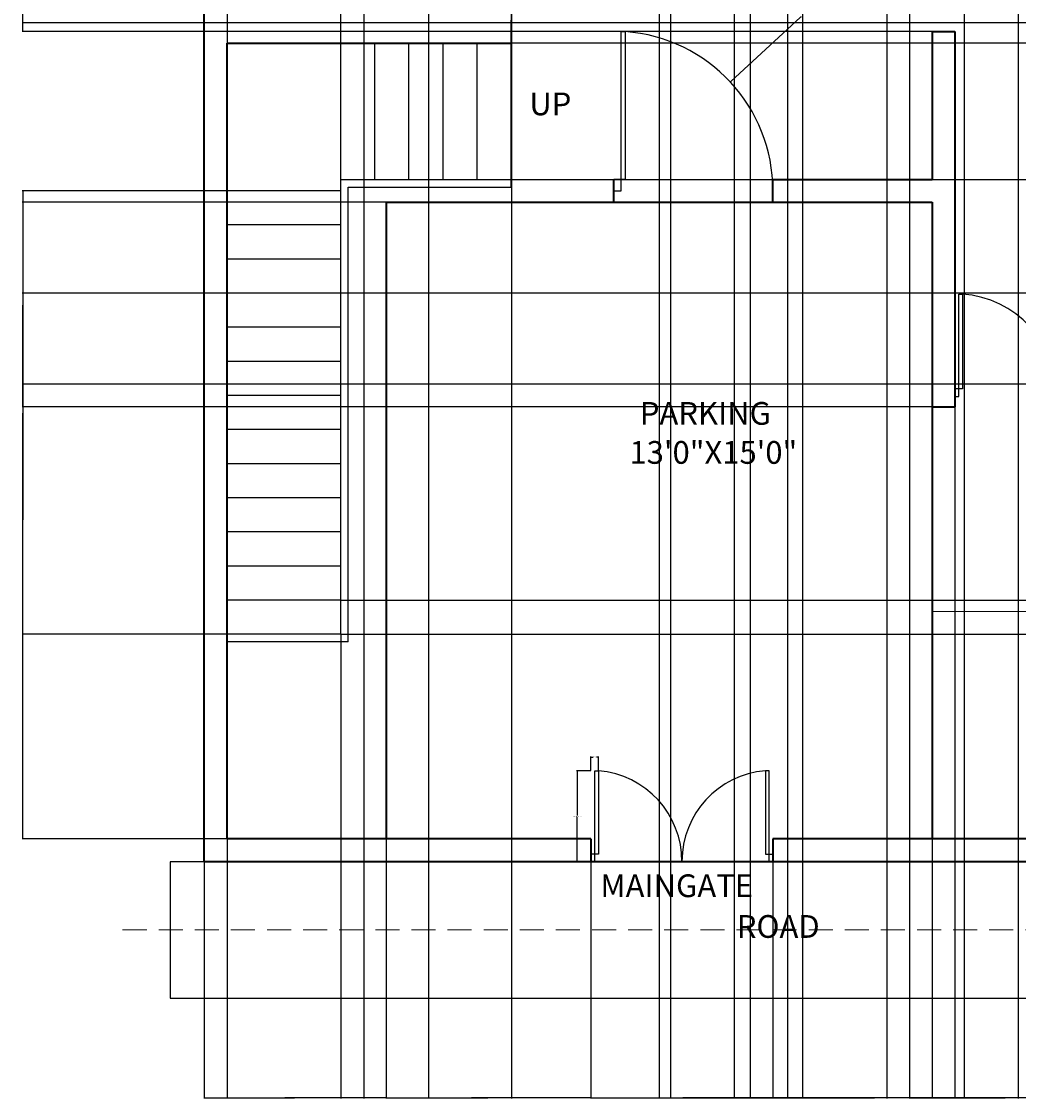
# Model space of a CAD drawing. Units: inches. Extents: x 2608 to 3003, y 1827 to 2396.
# Tile 1 of 5: x 2608 to 2871, y 1827 to 2111. Entities that reach past the tile are written whole.
import ezdxf

# ---------------------------------------------------------------- set-up
doc = ezdxf.new("R2010")
doc.units = ezdxf.units.IN
doc.linetypes.add('DASHED2', pattern=[9.525, 6.35, -3.175])
for name, color, linetype, lineweight in [('A-ANNO-DIMS', 2, 'Continuous', 18), ('A-ANNO-TEXT', 7, 'Continuous', 25), ('A-AREA-IDEN', 7, 'Continuous', 25), ('A-DOOR', 50, 'Continuous', 25), ('A-DOOR-GATE', 50, 'Continuous', 25), ('A-FLOR', 111, 'Continuous', 18), ('A-FLOR-STRS', 111, 'Continuous', 25), ('A-WALL', 111, 'Continuous', 35), ('C-ROAD', 111, 'Continuous', 25), ('C-ROAD-CNTR', 255, 'DASHED2', 18)]:
    doc.layers.add(name, color=color, linetype=linetype, lineweight=lineweight)
doc.styles.get("Standard").update_dxf_attribs({"font": 'arial.ttf'})
doc.dimstyles.get("Standard").update_dxf_attribs({"dimtxt": 0.18, "dimasz": 0.18, "dimexe": 0.18, "dimexo": 0.0625, "dimgap": 0.09, "dimtad": 0, "dimtih": 1, "dimtoh": 1, "dimdec": 4, "dimzin": 0, "dimdsep": 46, "dimtxsty": 'Standard', "dimcen": 0.09, "dimadec": 0, "dimazin": 0, "dimtfac": 1, "dimtdec": 4, "dimtofl": 0, "dimtmove": 0, "dimatfit": 3, "dimfxl": 1, "dimtolj": 1, "dimtzin": 0, "dimarcsym": 0})

# ---------------------------------------------------------------- blocks, each defined once
blk = doc.blocks.new('GATE-LEAF-24')
for p, q in [((1, 0), (1, 24)), ((1, 24), (2, 24)), ((2, 24), (2, 2)), ((2, 2), (0, 2)), ((0, 0), (1, 0))]:
    blk.add_line(p, q)
blk = doc.blocks.new('*D26')
at = {"layer": 'A-ANNO-DIMS', "color": 0, "lineweight": -2, "transparency": 16777216}
for p, q in [((2757.85, 1913.49), (2754.14, 1913.49)), ((2754.32, 1913.31), (2754.32, 1901.67)), ((2754.32, 1889.67), (2754.32, 1901.31)), ((2757.85, 1889.49), (2754.14, 1889.49))]:
    blk.add_line(p, q, dxfattribs=at)
at = {"layer": 'A-ANNO-DIMS', "color": 0, "transparency": 16777216}
for points in [[(2754.29, 1913.31), (2754.35, 1913.31), (2754.32, 1913.49)], [(2754.29, 1889.67), (2754.35, 1889.67), (2754.32, 1889.49)]]:
    blk.add_solid(points, dxfattribs=at)
at = {"layer": 'Defpoints', "color": 0, "transparency": 16777216}
for p in [(2754.32, 1913.49), (2757.92, 1913.49), (2757.92, 1889.49)]:
    blk.add_point(p, dxfattribs=at)
at = {"layer": 'A-ANNO-DIMS', "color": 0, "transparency": 16777216, "insert": (2754.32, 1901.49), "char_height": 0.18, "attachment_point": 5}
blk.add_mtext('\\A1;GATE LEAF 24 TYP.', dxfattribs=at)
blk = doc.blocks.new('*D27')
at = {"layer": 'A-ANNO-DIMS', "color": 0, "lineweight": -2, "transparency": 16777216}
for p, q in [((2757.92, 1913.55), (2757.92, 1917.27)), ((2758.1, 1917.09), (2758.46, 1917.09)), ((2759.74, 1917.09), (2759.38, 1917.09)), ((2759.92, 1913.55), (2759.92, 1917.27))]:
    blk.add_line(p, q, dxfattribs=at)
at = {"layer": 'A-ANNO-DIMS', "color": 0, "transparency": 16777216}
for points in [[(2758.1, 1917.12), (2758.1, 1917.06), (2757.92, 1917.09)], [(2759.74, 1917.12), (2759.74, 1917.06), (2759.92, 1917.09)]]:
    blk.add_solid(points, dxfattribs=at)
at = {"layer": 'Defpoints', "color": 0, "transparency": 16777216}
for p in [(2759.92, 1917.09), (2757.92, 1913.49), (2759.92, 1913.49)]:
    blk.add_point(p, dxfattribs=at)
at = {"layer": 'A-ANNO-DIMS', "color": 0, "transparency": 16777216, "insert": (2758.92, 1917.09), "char_height": 0.18, "attachment_point": 5}
blk.add_mtext('\\A1;2 TYP.', dxfattribs=at)
blk = doc.blocks.new('*D30')
at = {"layer": 'A-ANNO-DIMS', "color": 0, "lineweight": -2, "transparency": 16777216}
for p, q in [((2703.92, 1895.43), (2703.92, 1827.03)), ((2655.92, 1889.43), (2655.92, 1827.03)), ((2656.1, 1827.21), (2679.69, 1827.21)), ((2703.74, 1827.21), (2680.14, 1827.21))]:
    blk.add_line(p, q, dxfattribs=at)
at = {"layer": 'A-ANNO-DIMS', "color": 0, "transparency": 16777216}
for points in [[(2656.1, 1827.24), (2656.1, 1827.18), (2655.92, 1827.21)], [(2703.74, 1827.24), (2703.74, 1827.18), (2703.92, 1827.21)]]:
    blk.add_solid(points, dxfattribs=at)
at = {"layer": 'Defpoints', "color": 0, "transparency": 16777216}
for p in [(2703.92, 1895.49), (2655.92, 1889.49), (2703.92, 1827.21)]:
    blk.add_point(p, dxfattribs=at)
at = {"layer": 'A-ANNO-DIMS', "color": 0, "transparency": 16777216, "insert": (2679.92, 1827.21), "char_height": 0.18, "attachment_point": 5}
blk.add_mtext('\\A1;48', dxfattribs=at)
blk = doc.blocks.new('*D31')
at = {"layer": 'A-ANNO-DIMS', "color": 0, "lineweight": -2, "transparency": 16777216}
for p, q in [((2703.92, 1895.43), (2703.92, 1827.03)), ((2757.92, 1889.43), (2757.92, 1827.03)), ((2704.1, 1827.21), (2730.7, 1827.21)), ((2757.74, 1827.21), (2731.13, 1827.21))]:
    blk.add_line(p, q, dxfattribs=at)
at = {"layer": 'A-ANNO-DIMS', "color": 0, "transparency": 16777216}
for points in [[(2704.1, 1827.24), (2704.1, 1827.18), (2703.92, 1827.21)], [(2757.74, 1827.24), (2757.74, 1827.18), (2757.92, 1827.21)]]:
    blk.add_solid(points, dxfattribs=at)
at = {"layer": 'Defpoints', "color": 0, "transparency": 16777216}
for p in [(2703.92, 1895.49), (2757.92, 1889.49), (2757.92, 1827.21)]:
    blk.add_point(p, dxfattribs=at)
at = {"layer": 'A-ANNO-DIMS', "color": 0, "transparency": 16777216, "insert": (2730.92, 1827.21), "char_height": 0.18, "attachment_point": 5}
blk.add_mtext('\\A1;54', dxfattribs=at)
blk = doc.blocks.new('*D32')
at = {"layer": 'A-ANNO-DIMS', "color": 0, "lineweight": -2, "transparency": 16777216}
for p, q in [((2757.92, 1889.43), (2757.92, 1827.03)), ((2805.92, 1889.43), (2805.92, 1827.03)), ((2758.1, 1827.21), (2781.69, 1827.21)), ((2805.74, 1827.21), (2782.14, 1827.21))]:
    blk.add_line(p, q, dxfattribs=at)
at = {"layer": 'A-ANNO-DIMS', "color": 0, "transparency": 16777216}
for points in [[(2758.1, 1827.24), (2758.1, 1827.18), (2757.92, 1827.21)], [(2805.74, 1827.24), (2805.74, 1827.18), (2805.92, 1827.21)]]:
    blk.add_solid(points, dxfattribs=at)
at = {"layer": 'Defpoints', "color": 0, "transparency": 16777216}
for p in [(2757.92, 1889.49), (2805.92, 1889.49), (2805.92, 1827.21)]:
    blk.add_point(p, dxfattribs=at)
at = {"layer": 'A-ANNO-DIMS', "color": 0, "transparency": 16777216, "insert": (2781.92, 1827.21), "char_height": 0.18, "attachment_point": 5}
blk.add_mtext('\\A1;48', dxfattribs=at)
blk = doc.blocks.new('*D33')
at = {"layer": 'A-ANNO-DIMS', "color": 0, "lineweight": -2, "transparency": 16777216}
for p, q in [((2847.92, 1895.43), (2847.92, 1827.03)), ((2805.92, 1889.43), (2805.92, 1827.03)), ((2806.1, 1827.21), (2826.69, 1827.21)), ((2847.74, 1827.21), (2827.14, 1827.21))]:
    blk.add_line(p, q, dxfattribs=at)
at = {"layer": 'A-ANNO-DIMS', "color": 0, "transparency": 16777216}
for points in [[(2806.1, 1827.24), (2806.1, 1827.18), (2805.92, 1827.21)], [(2847.74, 1827.24), (2847.74, 1827.18), (2847.92, 1827.21)]]:
    blk.add_solid(points, dxfattribs=at)
at = {"layer": 'Defpoints', "color": 0, "transparency": 16777216}
for p in [(2847.92, 1895.49), (2805.92, 1889.49), (2847.92, 1827.21)]:
    blk.add_point(p, dxfattribs=at)
at = {"layer": 'A-ANNO-DIMS', "color": 0, "transparency": 16777216, "insert": (2826.92, 1827.21), "char_height": 0.18, "attachment_point": 5}
blk.add_mtext('\\A1;42', dxfattribs=at)
blk = doc.blocks.new('*D34')
at = {"layer": 'A-ANNO-DIMS', "color": 0, "lineweight": -2, "transparency": 16777216}
for p, q in [((2703.85, 2063.49), (2607.92, 2063.49)), ((2608.1, 2063.31), (2608.1, 1979.67)), ((2608.1, 1895.67), (2608.1, 1979.31)), ((2703.85, 1895.49), (2607.92, 1895.49))]:
    blk.add_line(p, q, dxfattribs=at)
at = {"layer": 'A-ANNO-DIMS', "color": 0, "transparency": 16777216}
for points in [[(2608.07, 2063.31), (2608.13, 2063.31), (2608.1, 2063.49)], [(2608.07, 1895.67), (2608.13, 1895.67), (2608.1, 1895.49)]]:
    blk.add_solid(points, dxfattribs=at)
at = {"layer": 'Defpoints', "color": 0, "transparency": 16777216}
for p in [(2608.1, 2063.49), (2703.92, 2063.49), (2703.92, 1895.49)]:
    blk.add_point(p, dxfattribs=at)
at = {"layer": 'A-ANNO-DIMS', "color": 0, "transparency": 16777216, "insert": (2608.1, 1979.49), "char_height": 0.18, "attachment_point": 5}
blk.add_mtext('\\A1;168', dxfattribs=at)
blk = doc.blocks.new('*D42')
at = {"layer": 'A-ANNO-DIMS', "color": 0, "lineweight": -2, "transparency": 16777216}
for p, q in [((2775.92, 2285.43), (2775.92, 1827.03)), ((2799.92, 2285.43), (2799.92, 1827.03)), ((2776.1, 1827.21), (2787.7, 1827.21)), ((2799.74, 1827.21), (2788.14, 1827.21))]:
    blk.add_line(p, q, dxfattribs=at)
at = {"layer": 'A-ANNO-DIMS', "color": 0, "transparency": 16777216}
for points in [[(2776.1, 1827.24), (2776.1, 1827.18), (2775.92, 1827.21)], [(2799.74, 1827.24), (2799.74, 1827.18), (2799.92, 1827.21)]]:
    blk.add_solid(points, dxfattribs=at)
at = {"layer": 'Defpoints', "color": 0, "transparency": 16777216}
for p in [(2775.92, 2285.49), (2799.92, 2285.49), (2799.92, 1827.21)]:
    blk.add_point(p, dxfattribs=at)
at = {"layer": 'A-ANNO-DIMS', "color": 0, "transparency": 16777216, "insert": (2787.92, 1827.21), "char_height": 0.18, "attachment_point": 5}
blk.add_mtext('\\A1;24', dxfattribs=at)
blk = doc.blocks.new('*D43')
at = {"layer": 'A-ANNO-DIMS', "color": 0, "lineweight": -2, "transparency": 16777216}
for p, q in [((2661.92, 2363.43), (2661.92, 1827.03)), ((2698.03, 2363.43), (2698.03, 1827.03)), ((2662.1, 1827.21), (2679.51, 1827.21)), ((2697.85, 1827.21), (2680.44, 1827.21))]:
    blk.add_line(p, q, dxfattribs=at)
at = {"layer": 'A-ANNO-DIMS', "color": 0, "transparency": 16777216}
for points in [[(2662.1, 1827.24), (2662.1, 1827.18), (2661.92, 1827.21)], [(2697.85, 1827.24), (2697.85, 1827.18), (2698.03, 1827.21)]]:
    blk.add_solid(points, dxfattribs=at)
at = {"layer": 'Defpoints', "color": 0, "transparency": 16777216}
for p in [(2661.92, 2363.49), (2698.03, 2363.49), (2698.03, 1827.21)]:
    blk.add_point(p, dxfattribs=at)
at = {"layer": 'A-ANNO-DIMS', "color": 0, "transparency": 16777216, "insert": (2679.97, 1827.21), "char_height": 0.18, "attachment_point": 5}
blk.add_mtext('\\A1;36.116', dxfattribs=at)
blk = doc.blocks.new('*D44')
at = {"layer": 'A-ANNO-DIMS', "color": 0, "lineweight": -2, "transparency": 16777216}
for p, q in [((2775.92, 2363.43), (2775.92, 1827.03)), ((2795.68, 2363.43), (2795.68, 1827.03)), ((2776.1, 1827.21), (2785.34, 1827.21)), ((2795.5, 1827.21), (2786.25, 1827.21))]:
    blk.add_line(p, q, dxfattribs=at)
at = {"layer": 'A-ANNO-DIMS', "color": 0, "transparency": 16777216}
for points in [[(2776.1, 1827.24), (2776.1, 1827.18), (2775.92, 1827.21)], [(2795.5, 1827.24), (2795.5, 1827.18), (2795.68, 1827.21)]]:
    blk.add_solid(points, dxfattribs=at)
at = {"layer": 'Defpoints', "color": 0, "transparency": 16777216}
for p in [(2775.92, 2363.49), (2795.68, 2363.49), (2795.68, 1827.21)]:
    blk.add_point(p, dxfattribs=at)
at = {"layer": 'A-ANNO-DIMS', "color": 0, "transparency": 16777216, "insert": (2785.8, 1827.21), "char_height": 0.18, "attachment_point": 5}
blk.add_mtext('\\A1;19.766', dxfattribs=at)
blk = doc.blocks.new('*D45')
at = {"layer": 'A-ANNO-DIMS', "color": 0, "lineweight": -2, "transparency": 16777216}
for p, q in [((2795.68, 2363.43), (2795.68, 1827.03)), ((2813.68, 2363.43), (2813.68, 1827.03)), ((2795.86, 1827.21), (2804.47, 1827.21)), ((2813.5, 1827.21), (2804.89, 1827.21))]:
    blk.add_line(p, q, dxfattribs=at)
at = {"layer": 'A-ANNO-DIMS', "color": 0, "transparency": 16777216}
for points in [[(2795.86, 1827.24), (2795.86, 1827.18), (2795.68, 1827.21)], [(2813.5, 1827.24), (2813.5, 1827.18), (2813.68, 1827.21)]]:
    blk.add_solid(points, dxfattribs=at)
at = {"layer": 'Defpoints', "color": 0, "transparency": 16777216}
for p in [(2795.68, 2363.49), (2813.68, 2363.49), (2813.68, 1827.21)]:
    blk.add_point(p, dxfattribs=at)
at = {"layer": 'A-ANNO-DIMS', "color": 0, "transparency": 16777216, "insert": (2804.68, 1827.21), "char_height": 0.18, "attachment_point": 5}
blk.add_mtext('\\A1;18', dxfattribs=at)
blk = doc.blocks.new('*D46')
at = {"layer": 'A-ANNO-DIMS', "color": 0, "lineweight": -2, "transparency": 16777216}
for p, q in [((2841.92, 2363.43), (2841.92, 1827.03)), ((2870.61, 2363.43), (2870.61, 1827.03)), ((2842.1, 1827.21), (2855.87, 1827.21)), ((2870.43, 1827.21), (2856.66, 1827.21))]:
    blk.add_line(p, q, dxfattribs=at)
at = {"layer": 'A-ANNO-DIMS', "color": 0, "transparency": 16777216}
for points in [[(2842.1, 1827.24), (2842.1, 1827.18), (2841.92, 1827.21)], [(2870.43, 1827.24), (2870.43, 1827.18), (2870.61, 1827.21)]]:
    blk.add_solid(points, dxfattribs=at)
at = {"layer": 'Defpoints', "color": 0, "transparency": 16777216}
for p in [(2841.92, 2363.49), (2870.61, 2363.49), (2870.61, 1827.21)]:
    blk.add_point(p, dxfattribs=at)
at = {"layer": 'A-ANNO-DIMS', "color": 0, "transparency": 16777216, "insert": (2856.26, 1827.21), "char_height": 0.18, "attachment_point": 5}
blk.add_mtext('\\A1;28.69', dxfattribs=at)
blk = doc.blocks.new('*D47')
at = {"layer": 'A-ANNO-DIMS', "color": 0, "lineweight": -2, "transparency": 16777216}
for p, q in [((2778.92, 2225.43), (2778.92, 1827.03)), ((2835.92, 2225.43), (2835.92, 1827.03)), ((2779.1, 1827.21), (2807.2, 1827.21)), ((2835.74, 1827.21), (2807.63, 1827.21))]:
    blk.add_line(p, q, dxfattribs=at)
at = {"layer": 'A-ANNO-DIMS', "color": 0, "transparency": 16777216}
for points in [[(2779.1, 1827.24), (2779.1, 1827.18), (2778.92, 1827.21)], [(2835.74, 1827.24), (2835.74, 1827.18), (2835.92, 1827.21)]]:
    blk.add_solid(points, dxfattribs=at)
at = {"layer": 'Defpoints', "color": 0, "transparency": 16777216}
for p in [(2778.92, 2225.49), (2835.92, 2225.49), (2835.92, 1827.21)]:
    blk.add_point(p, dxfattribs=at)
at = {"layer": 'A-ANNO-DIMS', "color": 0, "transparency": 16777216, "insert": (2807.42, 1827.21), "char_height": 0.18, "attachment_point": 5}
blk.add_mtext('\\A1;57', dxfattribs=at)
blk = doc.blocks.new('*D51')
at = {"layer": 'A-ANNO-DIMS', "color": 0, "lineweight": -2, "transparency": 16777216}
for p, q in [((2853.92, 2009.43), (2853.92, 1827.03)), ((2880.92, 2009.43), (2880.92, 1827.03)), ((2854.1, 1827.21), (2867.2, 1827.21)), ((2880.74, 1827.21), (2867.64, 1827.21))]:
    blk.add_line(p, q, dxfattribs=at)
at = {"layer": 'A-ANNO-DIMS', "color": 0, "transparency": 16777216}
for points in [[(2854.1, 1827.24), (2854.1, 1827.18), (2853.92, 1827.21)], [(2880.74, 1827.24), (2880.74, 1827.18), (2880.92, 1827.21)]]:
    blk.add_solid(points, dxfattribs=at)
at = {"layer": 'Defpoints', "color": 0, "transparency": 16777216}
for p in [(2853.92, 2009.49), (2880.92, 2009.49), (2880.92, 1827.21)]:
    blk.add_point(p, dxfattribs=at)
at = {"layer": 'A-ANNO-DIMS', "color": 0, "transparency": 16777216, "insert": (2867.42, 1827.21), "char_height": 0.18, "attachment_point": 5}
blk.add_mtext('\\A1;27', dxfattribs=at)
blk = doc.blocks.new('*D55')
at = {"layer": 'A-ANNO-DIMS', "color": 0, "lineweight": -2, "transparency": 16777216}
for p, q in [((2847.85, 2135.49), (2607.92, 2135.49)), ((2608.1, 2135.31), (2608.1, 2122.17)), ((2608.1, 2108.67), (2608.1, 2121.81)), ((2853.85, 2108.49), (2607.92, 2108.49))]:
    blk.add_line(p, q, dxfattribs=at)
at = {"layer": 'A-ANNO-DIMS', "color": 0, "transparency": 16777216}
for points in [[(2608.07, 2135.31), (2608.13, 2135.31), (2608.1, 2135.49)], [(2608.07, 2108.67), (2608.13, 2108.67), (2608.1, 2108.49)]]:
    blk.add_solid(points, dxfattribs=at)
at = {"layer": 'Defpoints', "color": 0, "transparency": 16777216}
for p in [(2608.1, 2135.49), (2847.92, 2135.49), (2853.92, 2108.49)]:
    blk.add_point(p, dxfattribs=at)
at = {"layer": 'A-ANNO-DIMS', "color": 0, "transparency": 16777216, "insert": (2608.1, 2121.99), "char_height": 0.18, "attachment_point": 5}
blk.add_mtext('\\A1;27', dxfattribs=at)
blk = doc.blocks.new('*D56')
at = {"layer": 'A-ANNO-DIMS', "color": 0, "lineweight": -2, "transparency": 16777216}
for p, q in [((2897.48, 2039.49), (2607.92, 2039.49)), ((2608.1, 2039.31), (2608.1, 2027.67)), ((2608.1, 2015.67), (2608.1, 2027.31)), ((2897.48, 2015.49), (2607.92, 2015.49))]:
    blk.add_line(p, q, dxfattribs=at)
at = {"layer": 'A-ANNO-DIMS', "color": 0, "transparency": 16777216}
for points in [[(2608.07, 2039.31), (2608.13, 2039.31), (2608.1, 2039.49)], [(2608.07, 2015.67), (2608.13, 2015.67), (2608.1, 2015.49)]]:
    blk.add_solid(points, dxfattribs=at)
at = {"layer": 'Defpoints', "color": 0, "transparency": 16777216}
for p in [(2608.1, 2039.49), (2897.55, 2039.49), (2897.55, 2015.49)]:
    blk.add_point(p, dxfattribs=at)
at = {"layer": 'A-ANNO-DIMS', "color": 0, "transparency": 16777216, "insert": (2608.1, 2027.49), "char_height": 0.18, "attachment_point": 5}
blk.add_mtext('\\A1;24', dxfattribs=at)
blk = doc.blocks.new('*D58')
at = {"layer": 'A-ANNO-DIMS', "color": 0, "lineweight": -2, "transparency": 16777216}
for p, q in [((2847.85, 2063.49), (2607.92, 2063.49)), ((2608.1, 2063.31), (2608.1, 2036.67)), ((2608.1, 2009.67), (2608.1, 2036.31)), ((2847.85, 2009.49), (2607.92, 2009.49))]:
    blk.add_line(p, q, dxfattribs=at)
at = {"layer": 'A-ANNO-DIMS', "color": 0, "transparency": 16777216}
for points in [[(2608.07, 2063.31), (2608.13, 2063.31), (2608.1, 2063.49)], [(2608.07, 2009.67), (2608.13, 2009.67), (2608.1, 2009.49)]]:
    blk.add_solid(points, dxfattribs=at)
at = {"layer": 'Defpoints', "color": 0, "transparency": 16777216}
for p in [(2608.1, 2063.49), (2847.92, 2063.49), (2847.92, 2009.49)]:
    blk.add_point(p, dxfattribs=at)
at = {"layer": 'A-ANNO-DIMS', "color": 0, "transparency": 16777216, "insert": (2608.1, 2036.49), "char_height": 0.18, "attachment_point": 5}
blk.add_mtext('\\A1;54', dxfattribs=at)
blk = doc.blocks.new('*D62')
at = {"layer": 'A-ANNO-DIMS', "color": 0, "lineweight": -2, "transparency": 16777216}
for p, q in [((2925.85, 2135.49), (2607.92, 2135.49)), ((2608.1, 2135.31), (2608.1, 2123.33)), ((2608.1, 2110.99), (2608.1, 2122.97)), ((2928.1, 2110.81), (2607.92, 2110.81))]:
    blk.add_line(p, q, dxfattribs=at)
at = {"layer": 'A-ANNO-DIMS', "color": 0, "transparency": 16777216}
for points in [[(2608.07, 2135.31), (2608.13, 2135.31), (2608.1, 2135.49)], [(2608.07, 2110.99), (2608.13, 2110.99), (2608.1, 2110.81)]]:
    blk.add_solid(points, dxfattribs=at)
at = {"layer": 'Defpoints', "color": 0, "transparency": 16777216}
for p in [(2925.92, 2135.49), (2608.1, 2110.81), (2928.16, 2110.81)]:
    blk.add_point(p, dxfattribs=at)
at = {"layer": 'A-ANNO-DIMS', "color": 0, "transparency": 16777216, "insert": (2608.1, 2123.15), "char_height": 0.18, "attachment_point": 5}
blk.add_mtext('\\A1;24.675', dxfattribs=at)
blk = doc.blocks.new('*D65')
at = {"layer": 'A-ANNO-DIMS', "color": 0, "lineweight": -2, "transparency": 16777216}
for p, q in [((2661.92, 1949.43), (2661.92, 1827.03)), ((2691.92, 1949.43), (2691.92, 1827.03)), ((2662.1, 1827.21), (2676.7, 1827.21)), ((2691.74, 1827.21), (2677.13, 1827.21))]:
    blk.add_line(p, q, dxfattribs=at)
at = {"layer": 'A-ANNO-DIMS', "color": 0, "transparency": 16777216}
for points in [[(2662.1, 1827.24), (2662.1, 1827.18), (2661.92, 1827.21)], [(2691.74, 1827.24), (2691.74, 1827.18), (2691.92, 1827.21)]]:
    blk.add_solid(points, dxfattribs=at)
at = {"layer": 'Defpoints', "color": 0, "transparency": 16777216}
for p in [(2661.92, 1949.49), (2691.92, 1949.49), (2691.92, 1827.21)]:
    blk.add_point(p, dxfattribs=at)
at = {"layer": 'A-ANNO-DIMS', "color": 0, "transparency": 16777216, "insert": (2676.92, 1827.21), "char_height": 0.18, "attachment_point": 5}
blk.add_mtext('\\A1;30', dxfattribs=at)
blk = doc.blocks.new('*D66')
at = {"layer": 'A-ANNO-DIMS', "color": 0, "lineweight": -2, "transparency": 16777216}
for p, q in [((2691.98, 1958.49), (3003.02, 1958.49)), ((3002.84, 1958.31), (3002.84, 1954.17)), ((3002.84, 1949.67), (3002.84, 1953.81)), ((2691.98, 1949.49), (3003.02, 1949.49))]:
    blk.add_line(p, q, dxfattribs=at)
at = {"layer": 'A-ANNO-DIMS', "color": 0, "transparency": 16777216}
for points in [[(3002.81, 1958.31), (3002.87, 1958.31), (3002.84, 1958.49)], [(3002.81, 1949.67), (3002.87, 1949.67), (3002.84, 1949.49)]]:
    blk.add_solid(points, dxfattribs=at)
at = {"layer": 'Defpoints', "color": 0, "transparency": 16777216}
for p in [(2691.92, 1958.49), (3002.84, 1958.49), (2691.92, 1949.49)]:
    blk.add_point(p, dxfattribs=at)
at = {"layer": 'A-ANNO-DIMS', "color": 0, "transparency": 16777216, "insert": (3002.84, 1953.99), "char_height": 0.18, "attachment_point": 5}
blk.add_mtext('\\A1;9', dxfattribs=at)
blk = doc.blocks.new('*D67')
at = {"layer": 'A-ANNO-DIMS', "color": 0, "lineweight": -2, "transparency": 16777216}
for p, q in [((2661.85, 2066.49), (2607.92, 2066.49)), ((2608.1, 2066.31), (2608.1, 2008.17)), ((2608.1, 1949.67), (2608.1, 2007.81)), ((2661.85, 1949.49), (2607.92, 1949.49))]:
    blk.add_line(p, q, dxfattribs=at)
at = {"layer": 'A-ANNO-DIMS', "color": 0, "transparency": 16777216}
for points in [[(2608.07, 2066.31), (2608.13, 2066.31), (2608.1, 2066.49)], [(2608.07, 1949.67), (2608.13, 1949.67), (2608.1, 1949.49)]]:
    blk.add_solid(points, dxfattribs=at)
at = {"layer": 'Defpoints', "color": 0, "transparency": 16777216}
for p in [(2608.1, 2066.49), (2661.92, 2066.49), (2661.92, 1949.49)]:
    blk.add_point(p, dxfattribs=at)
at = {"layer": 'A-ANNO-DIMS', "color": 0, "transparency": 16777216, "insert": (2608.1, 2007.99), "char_height": 0.18, "attachment_point": 5}
blk.add_mtext('\\A1;117', dxfattribs=at)
blk = doc.blocks.new('*D68')
at = {"layer": 'A-ANNO-DIMS', "color": 0, "lineweight": -2, "transparency": 16777216}
for p, q in [((2736.98, 2105.49), (3003.02, 2105.49)), ((3002.84, 2105.31), (3002.84, 2087.67)), ((3002.84, 2069.67), (3002.84, 2087.31)), ((2736.98, 2069.49), (3003.02, 2069.49))]:
    blk.add_line(p, q, dxfattribs=at)
at = {"layer": 'A-ANNO-DIMS', "color": 0, "transparency": 16777216}
for points in [[(3002.81, 2105.31), (3002.87, 2105.31), (3002.84, 2105.49)], [(3002.81, 2069.67), (3002.87, 2069.67), (3002.84, 2069.49)]]:
    blk.add_solid(points, dxfattribs=at)
at = {"layer": 'Defpoints', "color": 0, "transparency": 16777216}
for p in [(2736.92, 2105.49), (3002.84, 2105.49), (2736.92, 2069.49)]:
    blk.add_point(p, dxfattribs=at)
at = {"layer": 'A-ANNO-DIMS', "color": 0, "transparency": 16777216, "insert": (3002.84, 2087.49), "char_height": 0.18, "attachment_point": 5}
blk.add_mtext('\\A1;36', dxfattribs=at)
blk = doc.blocks.new('*D69')
at = {"layer": 'A-ANNO-DIMS', "color": 0, "lineweight": -2, "transparency": 16777216}
for p, q in [((2691.92, 2105.55), (2691.92, 2395.95)), ((2692.1, 2395.77), (2714.19, 2395.77)), ((2736.74, 2395.77), (2714.64, 2395.77)), ((2736.92, 2105.55), (2736.92, 2395.95))]:
    blk.add_line(p, q, dxfattribs=at)
at = {"layer": 'A-ANNO-DIMS', "color": 0, "transparency": 16777216}
for points in [[(2692.1, 2395.8), (2692.1, 2395.74), (2691.92, 2395.77)], [(2736.74, 2395.8), (2736.74, 2395.74), (2736.92, 2395.77)]]:
    blk.add_solid(points, dxfattribs=at)
at = {"layer": 'Defpoints', "color": 0, "transparency": 16777216}
for p in [(2736.92, 2395.77), (2691.92, 2105.49), (2736.92, 2105.49)]:
    blk.add_point(p, dxfattribs=at)
at = {"layer": 'A-ANNO-DIMS', "color": 0, "transparency": 16777216, "insert": (2714.42, 2395.77), "char_height": 0.18, "attachment_point": 5}
blk.add_mtext('\\A1;45', dxfattribs=at)
blk = doc.blocks.new('*D70')
at = {"layer": 'A-ANNO-DIMS', "color": 0, "lineweight": -2, "transparency": 16777216}
for p, q in [((2809.78, 2162.35), (2809.78, 1827.03)), ((2856.37, 2162.35), (2856.37, 1827.03)), ((2809.96, 1827.21), (2832.68, 1827.21)), ((2856.19, 1827.21), (2833.47, 1827.21))]:
    blk.add_line(p, q, dxfattribs=at)
at = {"layer": 'A-ANNO-DIMS', "color": 0, "transparency": 16777216}
for points in [[(2809.96, 1827.24), (2809.96, 1827.18), (2809.78, 1827.21)], [(2856.19, 1827.24), (2856.19, 1827.18), (2856.37, 1827.21)]]:
    blk.add_solid(points, dxfattribs=at)
at = {"layer": 'Defpoints', "color": 0, "transparency": 16777216}
for p in [(2809.78, 2162.41), (2856.37, 2162.41), (2856.37, 1827.21)]:
    blk.add_point(p, dxfattribs=at)
at = {"layer": 'A-ANNO-DIMS', "color": 0, "transparency": 16777216, "insert": (2833.07, 1827.21), "char_height": 0.18, "attachment_point": 5}
blk.add_mtext('\\A1;46.59', dxfattribs=at)
blk = doc.blocks.new('*D72')
at = {"layer": 'A-ANNO-DIMS', "color": 0, "lineweight": -2, "transparency": 16777216}
for p, q in [((2715.11, 2140.45), (2715.11, 1827.03)), ((2737, 2140.45), (2737, 1827.03)), ((2715.29, 1827.21), (2725.66, 1827.21)), ((2736.82, 1827.21), (2726.45, 1827.21))]:
    blk.add_line(p, q, dxfattribs=at)
at = {"layer": 'A-ANNO-DIMS', "color": 0, "transparency": 16777216}
for points in [[(2715.29, 1827.24), (2715.29, 1827.18), (2715.11, 1827.21)], [(2736.82, 1827.24), (2736.82, 1827.18), (2737, 1827.21)]]:
    blk.add_solid(points, dxfattribs=at)
at = {"layer": 'Defpoints', "color": 0, "transparency": 16777216}
for p in [(2715.11, 2140.51), (2737, 2140.51), (2737, 1827.21)]:
    blk.add_point(p, dxfattribs=at)
at = {"layer": 'A-ANNO-DIMS', "color": 0, "transparency": 16777216, "insert": (2726.06, 1827.21), "char_height": 0.18, "attachment_point": 5}
blk.add_mtext('\\A1;21.89', dxfattribs=at)
blk = doc.blocks.new('*D76')
at = {"layer": 'A-ANNO-DIMS', "color": 0, "lineweight": -2, "transparency": 16777216}
for p, q in [((2813.16, 2112.32), (2794.82, 2095.3)), ((2813.34, 2112.32), (2813.16, 2112.32)), ((2763.83, 2066.6), (2764.01, 2066.6)), ((2763.92, 2066.51), (2763.92, 2066.69))]:
    blk.add_line(p, q, dxfattribs=at)
at = {"layer": 'A-ANNO-DIMS', "color": 0, "transparency": 16777216}
blk.add_solid([(2794.8, 2095.32), (2794.85, 2095.28), (2794.69, 2095.18)], dxfattribs=at)
at = {"layer": 'Defpoints', "color": 0, "transparency": 16777216}
for p in [(2794.69, 2095.18), (2763.92, 2066.6)]:
    blk.add_point(p, dxfattribs=at)
at = {"layer": 'A-ANNO-DIMS', "color": 0, "transparency": 16777216, "insert": (2813.64, 2112.32), "char_height": 0.18, "attachment_point": 5}
blk.add_mtext('\\A1;R42', dxfattribs=at)

msp = doc.modelspace()

# ---------------------------------------------------------------- linework, layer by layer
at = {"layer": 'A-DOOR'}
for p, q in [((2765.9155, 2066.4896), (2765.9155, 2108.4896)), ((2765.9155, 2108.4896), (2766.9155, 2108.4896)), ((2766.9155, 2108.4896), (2766.9155, 2069.4896)), ((2766.9155, 2069.4896), (2763.9155, 2069.4896)), ((2763.9155, 2066.4896), (2765.9155, 2066.4896)), ((2854.9155, 2012.2489), (2854.9155, 2039.2489)), ((2854.9155, 2039.2489), (2855.9155, 2039.2489)), ((2855.9155, 2039.2489), (2855.9155, 2014.2489)), ((2855.9155, 2014.2489), (2853.9155, 2014.2489)), ((2853.9155, 2012.2489), (2854.9155, 2012.2489))]:
    msp.add_line(p, q, dxfattribs=at)
for centre, radius, start, end in [((2763.9157, 2066.5969), 42, 359.853664, 85.904144), ((2853.9161, 2012.323), 27, 0.353483, 85.753071)]:
    msp.add_arc(centre, radius, start, end, dxfattribs=at)
at = {"layer": 'A-DOOR-GATE'}
for centre, start, end in [((2757.9157, 1889.5731), 359.800738, 85.220156), ((2805.9157, 1889.5731), 94.78054, 180.000058)]:
    msp.add_arc(centre, 24, start, end, dxfattribs=at)
at = {"layer": 'A-FLOR'}
msp.add_line((2949.9155, 1955.4896), (2847.9155, 1955.4896), dxfattribs=at)
at = {"layer": 'A-FLOR-STRS'}
for p, q in [((2736.9155, 2067.4896), (2736.9155, 2111.4896)), ((2691.9155, 2069.4896), (2691.9155, 2105.4896)), ((2700.9155, 2069.4896), (2700.9155, 2105.4896)), ((2709.9155, 2069.4896), (2709.9155, 2105.4896)), ((2718.9155, 2069.4896), (2718.9155, 2105.4896)), ((2727.9155, 2069.4896), (2727.9155, 2105.4896)), ((2691.9155, 2069.4896), (2736.9155, 2069.4896)), ((2691.9155, 1949.4896), (2691.9155, 2069.4896)), ((2691.9155, 2066.4896), (2661.9155, 2066.4896)), ((2693.9155, 1947.4896), (2693.9155, 2067.4896)), ((2693.9155, 2067.4896), (2736.9155, 2067.4896)), ((2691.9155, 2057.4896), (2661.9155, 2057.4896)), ((2691.9155, 2048.4896), (2661.9155, 2048.4896)), ((2691.9155, 2039.4896), (2661.9155, 2039.4896)), ((2691.9155, 2030.4896), (2661.9155, 2030.4896)), ((2691.9155, 2021.4896), (2661.9155, 2021.4896)), ((2691.9155, 2012.4896), (2661.9155, 2012.4896)), ((2691.9155, 2003.4896), (2661.9155, 2003.4896)), ((2691.9155, 1994.4896), (2661.9155, 1994.4896)), ((2691.9155, 1985.4896), (2661.9155, 1985.4896)), ((2691.9155, 1976.4896), (2661.9155, 1976.4896)), ((2691.9155, 1967.4896), (2661.9155, 1967.4896)), ((2691.9155, 1958.4896), (2661.9155, 1958.4896)), ((2691.9155, 1949.4896), (2661.9155, 1949.4896)), ((2693.9155, 1947.4896), (2661.9155, 1947.4896))]:
    msp.add_line(p, q, dxfattribs=at)
at = {"layer": 'A-WALL'}
for p, q in [((2847.9155, 2108.4896), (2847.9155, 2069.4896)), ((2847.9155, 2108.4896), (2853.9155, 2108.4896)), ((2853.9155, 2108.4896), (2853.9155, 2009.4896)), ((2661.9155, 1895.4896), (2661.9155, 2105.4896)), ((2661.9155, 2105.4896), (2736.9155, 2105.4896)), ((2763.9155, 2063.4896), (2763.9155, 2069.4896)), ((2805.9155, 2063.4896), (2805.9155, 2069.4896)), ((2805.9155, 2069.4896), (2847.9155, 2069.4896)), ((2703.9155, 2063.4896), (2703.9155, 1895.4896)), ((2703.9155, 2063.4896), (2847.9155, 2063.4896)), ((2847.9155, 2063.4896), (2847.9155, 1895.4896)), ((2847.9155, 2009.4896), (2853.9155, 2009.4896)), ((2757.9155, 1895.4896), (2661.9155, 1895.4896)), ((2757.9155, 1895.4896), (2757.9155, 1889.4896)), ((2949.9155, 1895.4896), (2805.9155, 1895.4896)), ((2805.9155, 1895.4896), (2805.9155, 1889.4896))]:
    msp.add_line(p, q, dxfattribs=at)
msp.add_lwpolyline([(2655.9155, 2369.4896), (2955.9155, 2369.4896), (2955.9155, 1889.4896), (2655.9155, 1889.4896)], close=True, dxfattribs=at)
at = {"layer": 'C-ROAD'}
for p, q in [((2655.9155, 1889.4896), (2646.9155, 1889.4896)), ((2646.9155, 1889.4896), (2646.9155, 1853.4896)), ((2646.9155, 1853.4896), (2964.9155, 1853.4896))]:
    msp.add_line(p, q, dxfattribs=at)
at = {"layer": 'C-ROAD-CNTR'}
msp.add_line((2634.3755, 1871.4896), (2976.5614, 1871.4896), dxfattribs=at)

# ---------------------------------------------------------------- block references
at = {"layer": 'A-DOOR-GATE'}
msp.add_blockref('GATE-LEAF-24', (2757.916, 1889.49), dxfattribs=at)
at = {"layer": 'A-DOOR-GATE', "extrusion": (0, 0, -1), "zscale": -1}
msp.add_blockref('GATE-LEAF-24', (-2805.9151, 1889.49), dxfattribs=at)

# ---------------------------------------------------------------- texts
at = {"layer": 'A-ANNO-TEXT'}
for tag, p in [('UP', (2741.6582, 2086.4257)), ('MAINGATE', (2760.4126, 1880.1477)), ('ROAD', (2796.379, 1869.4051))]:
    msp.add_attdef(tag, p, '', height=6, dxfattribs=at)
at = {"layer": 'A-AREA-IDEN'}
for tag, p in [('PARKING', (2770.8037, 2004.7694)), ('13\'0"X15\'0"', (2768.0756, 1994.4722))]:
    msp.add_attdef(tag, p, '', height=6, dxfattribs=at)

# ---------------------------------------------------------------- dimensions: what is measured, and where the dimension line sits
at = {"layer": 'A-ANNO-DIMS'}
for base, p1, p2, override, picture, middle in [((2736.9155, 2395.7696), (2691.9155, 2105.4896), (2736.9155, 2105.4896), {"dimdec": 0, "dimlfac": 1, "dimrnd": 0, "dimzin": 0, "dimdsep": 46, "dimlunit": 2}, '*D69', (2714.4155, 2395.7696)), ((2698.0318, 1827.2096), (2661.9155, 2363.4896), (2698.0318, 2363.4896), {"dimdec": 3, "dimlfac": 1, "dimrnd": 0, "dimzin": 0, "dimdsep": 46, "dimlunit": 2}, '*D43', (2679.9737, 1827.2096)), ((2795.6817, 1827.2096), (2775.9155, 2363.4896), (2795.6817, 2363.4896), {"dimdec": 3, "dimlfac": 1, "dimrnd": 0, "dimzin": 0, "dimdsep": 46, "dimlunit": 2}, '*D44', (2785.7986, 1827.2096)), ((2813.6817, 1827.2096), (2795.6817, 2363.4896), (2813.6817, 2363.4896), {"dimdec": 0, "dimlfac": 1, "dimrnd": 0, "dimzin": 0, "dimdsep": 46, "dimlunit": 2}, '*D45', (2804.6817, 1827.2096)), ((2870.6078, 1827.2096), (2841.9155, 2363.4896), (2870.6078, 2363.4896), {"dimdec": 2, "dimlfac": 1, "dimrnd": 0, "dimzin": 0, "dimdsep": 46, "dimlunit": 2}, '*D46', (2856.2616, 1827.2096)), ((2799.9155, 1827.2096), (2775.9155, 2285.4896), (2799.9155, 2285.4896), {"dimdec": 0, "dimlfac": 1, "dimrnd": 0, "dimzin": 0, "dimdsep": 46, "dimlunit": 2}, '*D42', (2787.9155, 1827.2096)), ((2835.9155, 1827.2096), (2778.9155, 2225.4896), (2835.9155, 2225.4896), {"dimdec": 0, "dimlfac": 1, "dimrnd": 0, "dimzin": 0, "dimdsep": 46, "dimlunit": 2}, '*D47', (2807.4155, 1827.2096)), ((2856.3703, 1827.2096), (2809.7764, 2162.4082), (2856.3703, 2162.4082), {"dimdec": 2, "dimlfac": 1, "dimrnd": 0, "dimzin": 0, "dimdsep": 46, "dimlunit": 2}, '*D70', (2833.0733, 1827.2096)), ((2737.0038, 1827.2096), (2715.1137, 2140.51), (2737.0038, 2140.51), {"dimdec": 2, "dimlfac": 1, "dimrnd": 0, "dimzin": 0, "dimdsep": 46, "dimlunit": 2}, '*D72', (2726.0588, 1827.2096)), ((2880.9155, 1827.2096), (2853.9155, 2009.4896), (2880.9155, 2009.4896), {"dimdec": 0, "dimlfac": 1, "dimrnd": 0, "dimzin": 0, "dimdsep": 46, "dimlunit": 2}, '*D51', (2867.4155, 1827.2096)), ((2691.9155, 1827.2096), (2661.9155, 1949.4896), (2691.9155, 1949.4896), {"dimdec": 0, "dimlfac": 1, "dimrnd": 0, "dimzin": 0, "dimdsep": 46, "dimlunit": 2}, '*D65', (2676.9155, 1827.2096)), ((2703.9155, 1827.2096), (2655.9155, 1889.4896), (2703.9155, 1895.4896), {"dimdec": 0, "dimlfac": 1, "dimrnd": 0, "dimzin": 0, "dimdsep": 46, "dimlunit": 2}, '*D30', (2679.9155, 1827.2096)), ((2757.9155, 1827.2096), (2703.9155, 1895.4896), (2757.9155, 1889.4896), {"dimdec": 0, "dimlfac": 1, "dimrnd": 0, "dimzin": 0, "dimdsep": 46, "dimlunit": 2}, '*D31', (2730.9155, 1827.2096)), ((2847.9155, 1827.2096), (2805.9155, 1889.4896), (2847.9155, 1895.4896), {"dimdec": 0, "dimlfac": 1, "dimrnd": 0, "dimzin": 0, "dimdsep": 46, "dimlunit": 2}, '*D33', (2826.9155, 1827.2096)), ((2805.9155, 1827.2096), (2757.9155, 1889.4896), (2805.9155, 1889.4896), {"dimdec": 0, "dimlfac": 1, "dimrnd": 0, "dimzin": 0, "dimdsep": 46, "dimlunit": 2}, '*D32', (2781.9155, 1827.2096))]:
    dim = msp.add_linear_dim(base=base, p1=p1, p2=p2, dimstyle='Standard', override=override, dxfattribs=at)
    dim.commit()
    dim.dimension.update_dxf_attribs({"geometry": picture, "text_midpoint": middle})
for base, p1, p2, override, picture, middle in [((2608.0955, 2110.8146), (2925.9155, 2135.4896), (2928.1576, 2110.8146), {"dimdec": 3, "dimlfac": 1, "dimrnd": 0, "dimzin": 0, "dimdsep": 46, "dimlunit": 2}, '*D62', (2608.0955, 2123.1521)), ((2608.0955, 2135.4896), (2853.9155, 2108.4896), (2847.9155, 2135.4896), {"dimdec": 0, "dimlfac": 1, "dimrnd": 0, "dimzin": 0, "dimdsep": 46, "dimlunit": 2}, '*D55', (2608.0955, 2121.9896)), ((3002.8414, 2105.4896), (2736.9155, 2069.4896), (2736.9155, 2105.4896), {"dimdec": 0, "dimlfac": 1, "dimrnd": 0, "dimzin": 0, "dimdsep": 46, "dimlunit": 2}, '*D68', (3002.8414, 2087.4896)), ((2608.0955, 2066.4896), (2661.9155, 1949.4896), (2661.9155, 2066.4896), {"dimdec": 0, "dimlfac": 1, "dimrnd": 0, "dimzin": 0, "dimdsep": 46, "dimlunit": 2}, '*D67', (2608.0955, 2007.9896)), ((2608.0955, 2063.4896), (2703.9155, 1895.4896), (2703.9155, 2063.4896), {"dimdec": 0, "dimlfac": 1, "dimrnd": 0, "dimzin": 0, "dimdsep": 46, "dimlunit": 2}, '*D34', (2608.0955, 1979.4896)), ((2608.0955, 2063.4896), (2847.9155, 2009.4896), (2847.9155, 2063.4896), {"dimdec": 0, "dimlfac": 1, "dimrnd": 0, "dimzin": 0, "dimdsep": 46, "dimlunit": 2}, '*D58', (2608.0955, 2036.4896)), ((2608.0955, 2039.4896), (2897.5458, 2015.4896), (2897.5458, 2039.4896), {"dimdec": 0, "dimlfac": 1, "dimrnd": 0, "dimzin": 0, "dimdsep": 46, "dimlunit": 2}, '*D56', (2608.0955, 2027.4896)), ((3002.8414, 1958.4896), (2691.9155, 1949.4896), (2691.9155, 1958.4896), {"dimdec": 0, "dimlfac": 1, "dimrnd": 0, "dimzin": 0, "dimdsep": 46, "dimlunit": 2}, '*D66', (3002.8414, 1953.9896))]:
    dim = msp.add_linear_dim(base=base, p1=p1, p2=p2, angle=90, dimstyle='Standard', override=override, dxfattribs=at)
    dim.commit()
    dim.dimension.update_dxf_attribs({"geometry": picture, "text_midpoint": middle})
dim = msp.add_radius_dim(center=(2763.9157, 2066.5969), mpoint=(2794.6929, 2095.1759), dimstyle='Standard', override={"dimdec": 0, "dimlfac": 1, "dimrnd": 0, "dimzin": 0, "dimdsep": 46, "dimlunit": 2}, dxfattribs=at)
dim.commit()
dim.dimension.update_dxf_attribs({"geometry": '*D76', "text_midpoint": (2813.6434, 2112.3233), "dimtype": 164})
dim = msp.add_linear_dim(base=(2759.9155, 1917.0896), p1=(2757.9155, 1913.4896), p2=(2759.9155, 1913.4896), text='<> TYP.', dimstyle='Standard', override={"dimdec": 0, "dimlfac": 1, "dimrnd": 0, "dimzin": 0, "dimdsep": 46, "dimlunit": 2}, dxfattribs=at)
dim.commit()
dim.dimension.update_dxf_attribs({"geometry": '*D27', "text_midpoint": (2758.9155, 1917.0896)})
dim = msp.add_linear_dim(base=(2754.3155, 1913.4896), p1=(2757.9155, 1889.4896), p2=(2757.9155, 1913.4896), angle=90, text='GATE LEAF <> TYP.', dimstyle='Standard', override={"dimdec": 0, "dimlfac": 1, "dimrnd": 0, "dimzin": 0, "dimdsep": 46, "dimlunit": 2}, dxfattribs=at)
dim.commit()
dim.dimension.update_dxf_attribs({"geometry": '*D26', "text_midpoint": (2754.3155, 1901.4896)})

doc.saveas('drawing.dxf')
